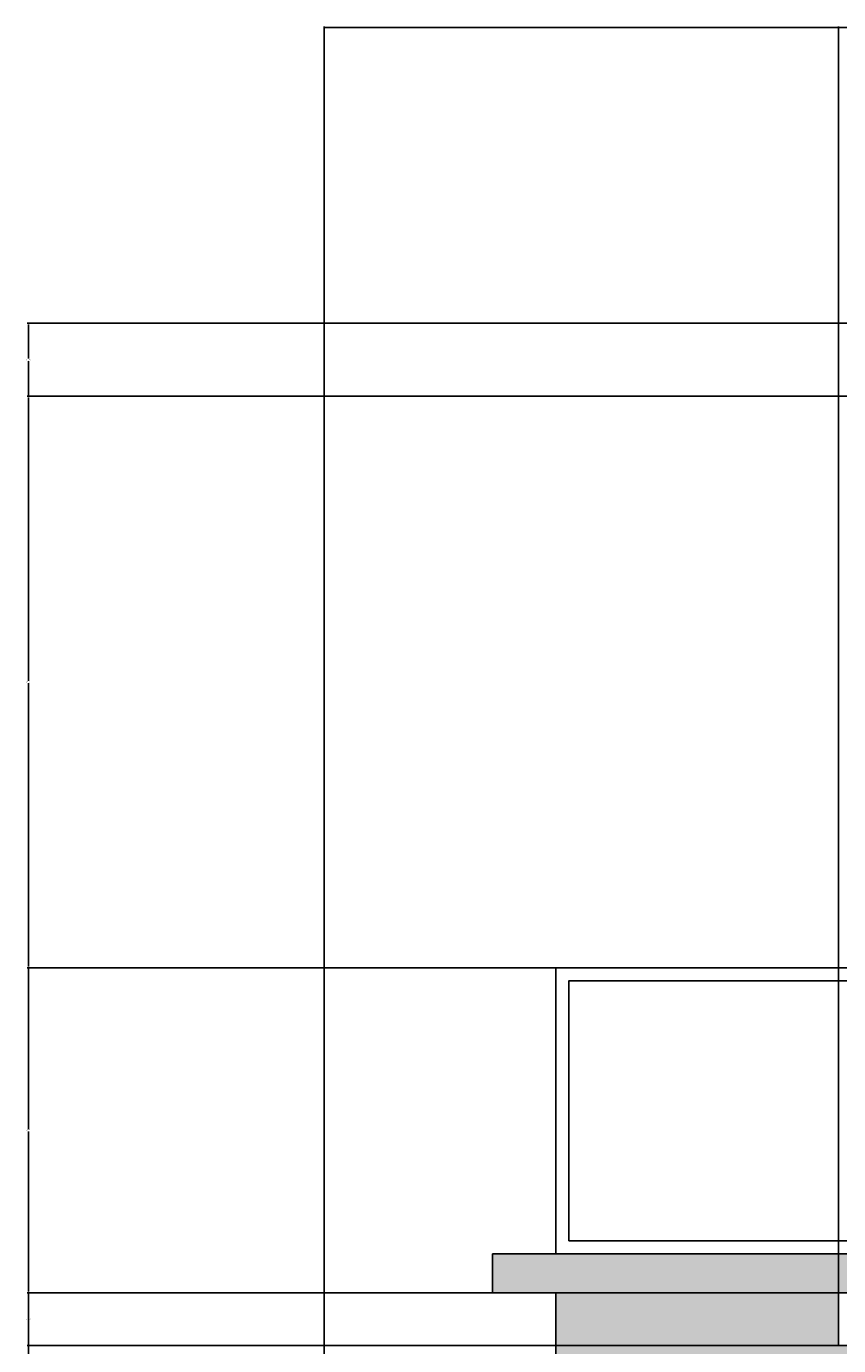
# Model space of a CAD drawing. Units: inches. Extents: x 3024 to 4744, y 1110 to 2100.
# Tile 24 of 29: x 3024 to 3149, y 1897 to 2100. Entities that reach past the tile are written whole.
import ezdxf

# ---------------------------------------------------------------- set-up
doc = ezdxf.new("R2010")
doc.units = ezdxf.units.IN
for name, color, linetype, lineweight in [('A-ANNO-DIMS', 2, 'Continuous', 18), ('A-ELEV', 7, 'Continuous', 25), ('A-ELEV-PATT', 252, 'Continuous', 13)]:
    doc.layers.add(name, color=color, linetype=linetype, lineweight=lineweight)
doc.styles.get("Standard").update_dxf_attribs({"font": 'arial.ttf'})
doc.dimstyles.get("Standard").update_dxf_attribs({"dimtxt": 0.18, "dimasz": 0.18, "dimexe": 0.18, "dimexo": 0.0625, "dimgap": 0.09, "dimtad": 0, "dimtih": 1, "dimtoh": 1, "dimdec": 1, "dimzin": 0, "dimdsep": 46, "dimlunit": 3, "dimtxsty": 'Standard', "dimcen": 0.09, "dimadec": 0, "dimazin": 0, "dimtfac": 1, "dimtdec": 1, "dimtofl": 0, "dimtmove": 0, "dimatfit": 3, "dimfxl": 1, "dimtolj": 1, "dimtzin": 0, "dimarcsym": 0})

# ---------------------------------------------------------------- blocks, each defined once
blk = doc.blocks.new('*D64')
at = {"layer": 'A-ANNO-DIMS', "color": 0, "lineweight": -2, "transparency": 16777216}
for p, q in [((3069.79, 1241.5), (3069.79, 2100.44)), ((3069.97, 2100.26), (3405.08, 2100.26)), ((3740.97, 2100.26), (3405.87, 2100.26)), ((3741.15, 1241.5), (3741.15, 2100.44))]:
    blk.add_line(p, q, dxfattribs=at)
at = {"layer": 'A-ANNO-DIMS', "color": 0, "transparency": 16777216}
for points in [[(3069.97, 2100.29), (3069.97, 2100.23), (3069.79, 2100.26)], [(3740.97, 2100.29), (3740.97, 2100.23), (3741.15, 2100.26)]]:
    blk.add_solid(points, dxfattribs=at)
at = {"layer": 'Defpoints', "color": 0, "transparency": 16777216}
for p in [(3741.15, 2100.26), (3069.79, 1241.43), (3741.15, 1241.43)]:
    blk.add_point(p, dxfattribs=at)
at = {"layer": 'A-ANNO-DIMS', "color": 0, "transparency": 16777216, "insert": (3405.47, 2100.26), "char_height": 0.18, "attachment_point": 5}
blk.add_mtext('\\A1;671.4', dxfattribs=at)
blk = doc.blocks.new('*D71')
at = {"layer": 'A-ANNO-DIMS', "color": 0, "lineweight": -2, "transparency": 16777216}
for p, q in [((3105.41, 1905.61), (3024.11, 1905.61)), ((3024.29, 1905.43), (3024.29, 1842.79)), ((3024.29, 1779.79), (3024.29, 1842.43)), ((3105.41, 1779.61), (3024.11, 1779.61))]:
    blk.add_line(p, q, dxfattribs=at)
at = {"layer": 'A-ANNO-DIMS', "color": 0, "transparency": 16777216}
for points in [[(3024.26, 1905.43), (3024.32, 1905.43), (3024.29, 1905.61)], [(3024.26, 1779.79), (3024.32, 1779.79), (3024.29, 1779.61)]]:
    blk.add_solid(points, dxfattribs=at)
at = {"layer": 'Defpoints', "color": 0, "transparency": 16777216}
for p in [(3024.29, 1905.61), (3105.47, 1905.61), (3105.47, 1779.61)]:
    blk.add_point(p, dxfattribs=at)
at = {"layer": 'A-ANNO-DIMS', "color": 0, "transparency": 16777216, "insert": (3024.29, 1842.61), "char_height": 0.18, "attachment_point": 5}
blk.add_mtext('\\A1;126', dxfattribs=at)
blk = doc.blocks.new('*D72')
at = {"layer": 'A-ANNO-DIMS', "color": 0, "lineweight": -2, "transparency": 16777216}
for p, q in [((3105.41, 1955.62), (3024.11, 1955.62)), ((3024.29, 1955.44), (3024.29, 1930.8)), ((3024.29, 1905.79), (3024.29, 1930.43)), ((3105.41, 1905.61), (3024.11, 1905.61))]:
    blk.add_line(p, q, dxfattribs=at)
at = {"layer": 'A-ANNO-DIMS', "color": 0, "transparency": 16777216}
for points in [[(3024.26, 1955.44), (3024.32, 1955.44), (3024.29, 1955.62)], [(3024.26, 1905.79), (3024.32, 1905.79), (3024.29, 1905.61)]]:
    blk.add_solid(points, dxfattribs=at)
at = {"layer": 'Defpoints', "color": 0, "transparency": 16777216}
for p in [(3024.29, 1955.62), (3105.47, 1955.62), (3105.47, 1905.61)]:
    blk.add_point(p, dxfattribs=at)
at = {"layer": 'A-ANNO-DIMS', "color": 0, "transparency": 16777216, "insert": (3024.29, 1930.62), "char_height": 0.18, "attachment_point": 5}
blk.add_mtext('\\A1;50.01', dxfattribs=at)
blk = doc.blocks.new('*D73')
at = {"layer": 'A-ANNO-DIMS', "color": 0, "lineweight": -2, "transparency": 16777216}
for p, q in [((3329.64, 2043.53), (3024.11, 2043.53)), ((3024.29, 2043.35), (3024.29, 1999.76)), ((3024.29, 1955.8), (3024.29, 1999.39)), ((3105.41, 1955.62), (3024.11, 1955.62))]:
    blk.add_line(p, q, dxfattribs=at)
at = {"layer": 'A-ANNO-DIMS', "color": 0, "transparency": 16777216}
for points in [[(3024.26, 2043.35), (3024.32, 2043.35), (3024.29, 2043.53)], [(3024.26, 1955.8), (3024.32, 1955.8), (3024.29, 1955.62)]]:
    blk.add_solid(points, dxfattribs=at)
at = {"layer": 'Defpoints', "color": 0, "transparency": 16777216}
for p in [(3024.29, 2043.53), (3329.7, 2043.53), (3105.47, 1955.62)]:
    blk.add_point(p, dxfattribs=at)
at = {"layer": 'A-ANNO-DIMS', "color": 0, "transparency": 16777216, "insert": (3024.29, 1999.57), "char_height": 0.18, "attachment_point": 5}
blk.add_mtext('\\A1;87.91', dxfattribs=at)
blk = doc.blocks.new('*D74')
at = {"layer": 'A-ANNO-DIMS', "color": 0, "lineweight": -2, "transparency": 16777216}
for p, q in [((3320.5, 2054.76), (3024.11, 2054.76)), ((3024.29, 2054.58), (3024.29, 2049.33)), ((3024.29, 2043.71), (3024.29, 2048.96)), ((3320.5, 2043.53), (3024.11, 2043.53))]:
    blk.add_line(p, q, dxfattribs=at)
at = {"layer": 'A-ANNO-DIMS', "color": 0, "transparency": 16777216}
for points in [[(3024.26, 2054.58), (3024.32, 2054.58), (3024.29, 2054.76)], [(3024.26, 2043.71), (3024.32, 2043.71), (3024.29, 2043.53)]]:
    blk.add_solid(points, dxfattribs=at)
at = {"layer": 'Defpoints', "color": 0, "transparency": 16777216}
for p in [(3024.29, 2054.76), (3320.57, 2054.76), (3320.57, 2043.53)]:
    blk.add_point(p, dxfattribs=at)
at = {"layer": 'A-ANNO-DIMS', "color": 0, "transparency": 16777216, "insert": (3024.29, 2049.14), "char_height": 0.18, "attachment_point": 5}
blk.add_mtext('\\A1;11.23', dxfattribs=at)
blk = doc.blocks.new('*D82')
at = {"layer": 'A-ANNO-DIMS', "color": 0, "lineweight": -2, "transparency": 16777216}
for p, q in [((3148.97, 1897.55), (3148.97, 2100.44)), ((3149.15, 2100.26), (3151.26, 2100.26)), ((3154.15, 2100.26), (3152.04, 2100.26)), ((3154.33, 1897.55), (3154.33, 2100.44))]:
    blk.add_line(p, q, dxfattribs=at)
at = {"layer": 'A-ANNO-DIMS', "color": 0, "transparency": 16777216}
for points in [[(3149.15, 2100.29), (3149.15, 2100.23), (3148.97, 2100.26)], [(3154.15, 2100.29), (3154.15, 2100.23), (3154.33, 2100.26)]]:
    blk.add_solid(points, dxfattribs=at)
at = {"layer": 'Defpoints', "color": 0, "transparency": 16777216}
for p in [(3154.33, 2100.26), (3148.97, 1897.49), (3154.33, 1897.49)]:
    blk.add_point(p, dxfattribs=at)
at = {"layer": 'A-ANNO-DIMS', "color": 0, "transparency": 16777216, "insert": (3151.65, 2100.26), "char_height": 0.18, "attachment_point": 5}
blk.add_mtext('\\A1;5.359', dxfattribs=at)
blk = doc.blocks.new('*D98')
at = {"layer": 'A-ANNO-DIMS', "color": 0, "lineweight": -2, "transparency": 16777216}
for p, q in [((3154.27, 1897.49), (3024.11, 1897.49)), ((3024.29, 1897.31), (3024.29, 1852.36)), ((3024.29, 1807.05), (3024.29, 1852)), ((3154.27, 1806.87), (3024.11, 1806.87))]:
    blk.add_line(p, q, dxfattribs=at)
at = {"layer": 'A-ANNO-DIMS', "color": 0, "transparency": 16777216}
for points in [[(3024.26, 1897.31), (3024.32, 1897.31), (3024.29, 1897.49)], [(3024.26, 1807.05), (3024.32, 1807.05), (3024.29, 1806.87)]]:
    blk.add_solid(points, dxfattribs=at)
at = {"layer": 'Defpoints', "color": 0, "transparency": 16777216}
for p in [(3024.29, 1897.49), (3154.33, 1897.49), (3154.33, 1806.87)]:
    blk.add_point(p, dxfattribs=at)
at = {"layer": 'A-ANNO-DIMS', "color": 0, "transparency": 16777216, "insert": (3024.29, 1852.18), "char_height": 0.18, "attachment_point": 5}
blk.add_mtext('\\A1;90.62', dxfattribs=at)
blk = doc.blocks.new('*D99')
at = {"layer": 'A-ANNO-DIMS', "color": 0, "lineweight": -2, "transparency": 16777216}
for p, q in [((3148.91, 1905.61), (3024.11, 1905.61)), ((3024.29, 1905.43), (3024.29, 1901.73)), ((3024.29, 1897.67), (3024.29, 1901.37)), ((3148.91, 1897.49), (3024.11, 1897.49))]:
    blk.add_line(p, q, dxfattribs=at)
at = {"layer": 'A-ANNO-DIMS', "color": 0, "transparency": 16777216}
for points in [[(3024.26, 1905.43), (3024.32, 1905.43), (3024.29, 1905.61)], [(3024.26, 1897.67), (3024.32, 1897.67), (3024.29, 1897.49)]]:
    blk.add_solid(points, dxfattribs=at)
at = {"layer": 'Defpoints', "color": 0, "transparency": 16777216}
for p in [(3024.29, 1905.61), (3148.97, 1905.61), (3148.97, 1897.49)]:
    blk.add_point(p, dxfattribs=at)
at = {"layer": 'A-ANNO-DIMS', "color": 0, "transparency": 16777216, "insert": (3024.29, 1901.55), "char_height": 0.18, "attachment_point": 5}
blk.add_mtext('\\A1;8.123', dxfattribs=at)

msp = doc.modelspace()

# ---------------------------------------------------------------- hatches: boundary and pattern name
at = {"layer": 'A-ELEV-PATT'}
h = msp.add_hatch(color=256, dxfattribs=at)
h.dxf.hatch_style = 1
h.paths.add_polyline_path([(3329.7033, 1407.6112), (3105.4722, 1407.6112), (3105.4722, 1401.6112), (3329.7033, 1401.6112)])
h.paths.add_polyline_path([(3329.7033, 1281.6112), (3105.4722, 1281.6112), (3105.4722, 1275.6112), (3112.3838, 1275.6112), (3329.7033, 1275.6112)])
h.paths.add_polyline_path([(3329.7033, 1533.6112), (3105.4722, 1533.6112), (3105.4722, 1527.6112), (3329.7033, 1527.6112)])
h.paths.add_polyline_path([(3329.7033, 1659.6112), (3105.4722, 1659.6112), (3105.4722, 1653.6112), (3329.7033, 1653.6112)])
h.paths.add_polyline_path([(3329.7033, 1785.6112), (3105.4722, 1785.6112), (3105.4722, 1779.6112), (3329.7033, 1779.6112)])
h.paths.add_polyline_path([(3329.7033, 1911.6112), (3105.4722, 1911.6112), (3095.7158, 1911.6112), (3095.7158, 1905.6112), (3329.7033, 1905.6112)])
h.paths.add_polyline_path([(3715.2286, 1911.6112), (3705.4722, 1911.6112), (3705.4722, 1905.6112), (3715.2286, 1905.6112)])
h.paths.add_polyline_path([(3688.5588, 1911.6112), (3481.2411, 1911.6112), (3481.2411, 1905.6112), (3688.5588, 1905.6112)])
h = msp.add_hatch(color=256, dxfattribs=at)
h.dxf.hatch_style = 1
h.paths.add_polyline_path([(3154.3287, 1897.4879), (3148.9694, 1897.4879), (3148.9694, 1905.6112), (3105.4722, 1905.6112), (3105.4722, 1785.6112), (3148.9694, 1785.6112), (3148.9694, 1795.0431), (3151.6604, 1795.0431), (3151.6604, 1806.8674), (3154.3287, 1806.8674)])
h.paths.add_polyline_path([(3329.7033, 1905.6112), (3292.6051, 1905.6112), (3292.6051, 1897.4879), (3287.2458, 1897.4879), (3287.2458, 1806.8674), (3288.3759, 1806.8674), (3288.3759, 1795.0431), (3292.6051, 1795.0431), (3292.6051, 1785.6112), (3329.7033, 1785.6112)])
h.paths.add_polyline_path([(3154.3287, 1771.4879), (3148.9694, 1771.4879), (3148.9694, 1779.6112), (3105.4722, 1779.6112), (3105.4722, 1659.6112), (3148.9694, 1659.6112), (3148.9694, 1669.0431), (3151.6604, 1669.0431), (3151.6604, 1680.8674), (3154.3287, 1680.8674)])
h.paths.add_polyline_path([(3329.7033, 1779.6112), (3292.6051, 1779.6112), (3292.6051, 1771.4879), (3287.2458, 1771.4879), (3287.2458, 1680.8674), (3288.3759, 1680.8674), (3288.3759, 1669.0431), (3292.6051, 1669.0431), (3292.6051, 1659.6112), (3329.7033, 1659.6112)])
h.paths.add_polyline_path([(3154.3287, 1645.4879), (3148.9694, 1645.4879), (3148.9694, 1653.6112), (3105.4722, 1653.6112), (3105.4722, 1533.6112), (3148.9694, 1533.6112), (3148.9694, 1543.0431), (3151.6604, 1543.0431), (3151.6604, 1554.8674), (3154.3287, 1554.8674)])
h.paths.add_polyline_path([(3329.7033, 1653.6112), (3292.6051, 1653.6112), (3292.6051, 1645.4879), (3287.2458, 1645.4879), (3287.2458, 1554.8674), (3288.3759, 1554.8674), (3288.3759, 1543.0431), (3292.6051, 1543.0431), (3292.6051, 1533.6112), (3329.7033, 1533.6112)])
h.paths.add_polyline_path([(3329.7033, 1527.6112), (3292.6051, 1527.6112), (3292.6051, 1519.4879), (3287.2458, 1519.4879), (3287.2458, 1428.8674), (3288.3759, 1428.8674), (3288.3759, 1417.0431), (3292.6051, 1417.0431), (3292.6051, 1407.6112), (3329.7033, 1407.6112)])
h.paths.add_polyline_path([(3329.7033, 1401.6112), (3292.6051, 1401.6112), (3292.6051, 1393.4879), (3287.2458, 1393.4879), (3287.2458, 1302.8674), (3288.3759, 1302.8674), (3288.3759, 1291.0431), (3292.6051, 1291.0431), (3292.6051, 1281.6112), (3329.7033, 1281.6112)])
h.paths.add_polyline_path([(3154.3287, 1393.4879), (3148.9694, 1393.4879), (3148.9694, 1401.6112), (3105.4722, 1401.6112), (3105.4722, 1281.6112), (3148.9694, 1281.6112), (3148.9694, 1291.0431), (3151.6604, 1291.0431), (3151.6604, 1302.8674), (3154.3287, 1302.8674)])
h.paths.add_polyline_path([(3154.3287, 1519.4879), (3148.9694, 1519.4879), (3148.9694, 1527.6112), (3105.4722, 1527.6112), (3105.4722, 1407.6112), (3148.9694, 1407.6112), (3148.9694, 1417.0431), (3151.6604, 1417.0431), (3151.6604, 1428.8674), (3154.3287, 1428.8674)])
h.paths.add_polyline_path([(3515.7606, 1897.4879), (3510.4013, 1897.4879), (3510.4013, 1905.6112), (3481.2411, 1905.6112), (3481.2411, 1785.6112), (3510.4013, 1785.6112), (3510.4013, 1795.0431), (3513.0923, 1795.0431), (3513.0923, 1806.8674), (3515.7606, 1806.8674)])
h.paths.add_polyline_path([(3688.5588, 1905.6112), (3654.037, 1905.6112), (3654.037, 1897.4879), (3648.6777, 1897.4879), (3648.6777, 1806.8674), (3649.8078, 1806.8674), (3649.8078, 1795.0431), (3654.037, 1795.0431), (3654.037, 1785.6112), (3688.5588, 1785.6112)])
h.paths.add_polyline_path([(3515.7606, 1771.4879), (3510.4013, 1771.4879), (3510.4013, 1779.6112), (3481.2411, 1779.6112), (3481.2411, 1659.6112), (3510.4013, 1659.6112), (3510.4013, 1669.0431), (3513.0923, 1669.0431), (3513.0923, 1680.8674), (3515.7606, 1680.8674)])
h.paths.add_polyline_path([(3688.5588, 1779.6112), (3654.037, 1779.6112), (3654.037, 1771.4879), (3648.6777, 1771.4879), (3648.6777, 1680.8674), (3649.8078, 1680.8674), (3649.8078, 1669.0431), (3654.037, 1669.0431), (3654.037, 1659.6112), (3688.5588, 1659.6112)])
h.paths.add_polyline_path([(3515.7606, 1645.4879), (3510.4013, 1645.4879), (3510.4013, 1653.6112), (3481.2411, 1653.6112), (3481.2411, 1533.6112), (3510.4013, 1533.6112), (3510.4013, 1543.0431), (3513.0923, 1543.0431), (3513.0923, 1554.8674), (3515.7606, 1554.8674)])
h.paths.add_polyline_path([(3688.5588, 1653.6112), (3654.037, 1653.6112), (3654.037, 1645.4879), (3648.6777, 1645.4879), (3648.6777, 1554.8674), (3649.8078, 1554.8674), (3649.8078, 1543.0431), (3654.037, 1543.0431), (3654.037, 1533.6112), (3688.5588, 1533.6112)])
h.paths.add_polyline_path([(3515.7606, 1519.4879), (3510.4013, 1519.4879), (3510.4013, 1527.6112), (3481.2411, 1527.6112), (3481.2411, 1407.6112), (3510.4013, 1407.6112), (3510.4013, 1417.0431), (3513.0923, 1417.0431), (3513.0923, 1428.8674), (3515.7606, 1428.8674)])
h.paths.add_polyline_path([(3688.5588, 1527.6112), (3654.037, 1527.6112), (3654.037, 1519.4879), (3648.6777, 1519.4879), (3648.6777, 1428.8674), (3649.8078, 1428.8674), (3649.8078, 1417.0431), (3654.037, 1417.0431), (3654.037, 1407.6112), (3688.5588, 1407.6112)])
h.paths.add_polyline_path([(3515.7606, 1393.4879), (3510.4013, 1393.4879), (3510.4013, 1401.6112), (3481.2411, 1401.6112), (3481.2411, 1281.6112), (3510.4013, 1281.6112), (3510.4013, 1291.0431), (3513.0923, 1291.0431), (3513.0923, 1302.8674), (3515.7606, 1302.8674)])
h.paths.add_polyline_path([(3688.5588, 1401.6112), (3654.037, 1401.6112), (3654.037, 1393.4879), (3648.6777, 1393.4879), (3648.6777, 1302.8674), (3649.8078, 1302.8674), (3649.8078, 1291.0431), (3654.037, 1291.0431), (3654.037, 1281.6112), (3688.5588, 1281.6112)])
h.paths.add_polyline_path([(3515.7606, 1267.4879), (3510.4013, 1267.4879), (3510.4013, 1275.6112), (3481.2411, 1275.6112), (3481.2411, 1155.6112), (3510.4013, 1155.6112), (3510.4013, 1165.0431), (3513.0923, 1165.0431), (3513.0923, 1176.8674), (3515.7606, 1176.8674)])
h.paths.add_polyline_path([(3688.5588, 1275.6112), (3654.037, 1275.6112), (3654.037, 1267.4879), (3648.6777, 1267.4879), (3648.6777, 1176.8674), (3649.8078, 1176.8674), (3649.8078, 1165.0431), (3654.037, 1165.0431), (3654.037, 1155.6112), (3688.5588, 1155.6112)])
h.paths.add_polyline_path([(3112.3838, 1275.6112), (3105.4722, 1275.6112), (3105.4722, 1171.0239), (3112.3838, 1171.0239)])

# ---------------------------------------------------------------- linework, layer by layer
at = {"layer": 'A-ELEV'}
for p, q in [((3095.7158, 1911.6112), (3329.7033, 1911.6112)), ((3095.7158, 1911.6112), (3329.7033, 1911.6112)), ((3105.4722, 1171.0239), (3105.4722, 1905.6112)), ((3329.7033, 1905.6112), (3105.4722, 1905.6112)), ((3105.4722, 1171.0239), (3105.4722, 1905.6112)), ((3329.7033, 1905.6112), (3105.4722, 1905.6112))]:
    msp.add_line(p, q, dxfattribs=at)
for points in [[(3329.7033, 1955.6193), (3105.4722, 1955.6193), (3105.4722, 1911.6112), (3329.7033, 1911.6112)], [(3329.7033, 1955.6193), (3105.4722, 1955.6193), (3105.4722, 1911.6112), (3329.7033, 1911.6112)], [(3329.7033, 1953.6193), (3107.4722, 1953.6193), (3107.4722, 1913.6112), (3329.7033, 1913.6112)], [(3329.7033, 1953.6193), (3107.4722, 1953.6193), (3107.4722, 1913.6112), (3329.7033, 1913.6112)], [(3095.7158, 1911.6112), (3095.7158, 1905.6112), (3329.7033, 1905.6112), (3329.7033, 1911.6112)], [(3095.7158, 1911.6112), (3095.7158, 1905.6112), (3329.7033, 1905.6112), (3329.7033, 1911.6112)]]:
    msp.add_lwpolyline(points, dxfattribs=at)

# ---------------------------------------------------------------- dimensions: what is measured, and where the dimension line sits
at = {"layer": 'A-ANNO-DIMS'}
for base, p1, p2, override, picture, middle in [((3741.1507, 2100.2584), (3069.7937, 1241.4341), (3741.1507, 1241.4341), {"dimdec": 1, "dimlfac": 1, "dimrnd": 0, "dimzin": 0, "dimdsep": 46, "dimlunit": 2}, '*D64', (3405.4722, 2100.2584)), ((3154.3287, 2100.2584), (3148.9694, 1897.4879), (3154.3287, 1897.4879), {"dimdec": 3, "dimlfac": 1, "dimrnd": 0, "dimzin": 0, "dimdsep": 46, "dimlunit": 2}, '*D82', (3151.6491, 2100.2584))]:
    dim = msp.add_linear_dim(base=base, p1=p1, p2=p2, dimstyle='Standard', override=override, dxfattribs=at)
    dim.commit()
    dim.dimension.update_dxf_attribs({"geometry": picture, "text_midpoint": middle})
for base, p1, p2, override, picture, middle in [((3024.2937, 2054.7584), (3320.5658, 2043.5286), (3320.5658, 2054.7584), {"dimdec": 2, "dimlfac": 1, "dimrnd": 0, "dimzin": 0, "dimdsep": 46, "dimlunit": 2}, '*D74', (3024.2937, 2049.1435)), ((3024.2937, 2043.5286), (3105.4722, 1955.6193), (3329.7033, 2043.5286), {"dimdec": 2, "dimlfac": 1, "dimrnd": 0, "dimzin": 0, "dimdsep": 46, "dimlunit": 2}, '*D73', (3024.2937, 1999.5739)), ((3024.2937, 1955.6193), (3105.4722, 1905.6112), (3105.4722, 1955.6193), {"dimdec": 2, "dimlfac": 1, "dimrnd": 0, "dimzin": 0, "dimdsep": 46, "dimlunit": 2}, '*D72', (3024.2937, 1930.6152)), ((3024.2937, 1905.6112), (3148.9694, 1897.4879), (3148.9694, 1905.6112), {"dimdec": 3, "dimlfac": 1, "dimrnd": 0, "dimzin": 0, "dimdsep": 46, "dimlunit": 2}, '*D99', (3024.2937, 1901.5495)), ((3024.2937, 1905.6112), (3105.4722, 1779.6112), (3105.4722, 1905.6112), {"dimdec": 0, "dimlfac": 1, "dimrnd": 0, "dimzin": 0, "dimdsep": 46, "dimlunit": 2}, '*D71', (3024.2937, 1842.6112)), ((3024.2937, 1897.4879), (3154.3287, 1806.8674), (3154.3287, 1897.4879), {"dimdec": 2, "dimlfac": 1, "dimrnd": 0, "dimzin": 0, "dimdsep": 46, "dimlunit": 2}, '*D98', (3024.2937, 1852.1776))]:
    dim = msp.add_linear_dim(base=base, p1=p1, p2=p2, angle=90, dimstyle='Standard', override=override, dxfattribs=at)
    dim.commit()
    dim.dimension.update_dxf_attribs({"geometry": picture, "text_midpoint": middle})

doc.saveas('drawing.dxf')
